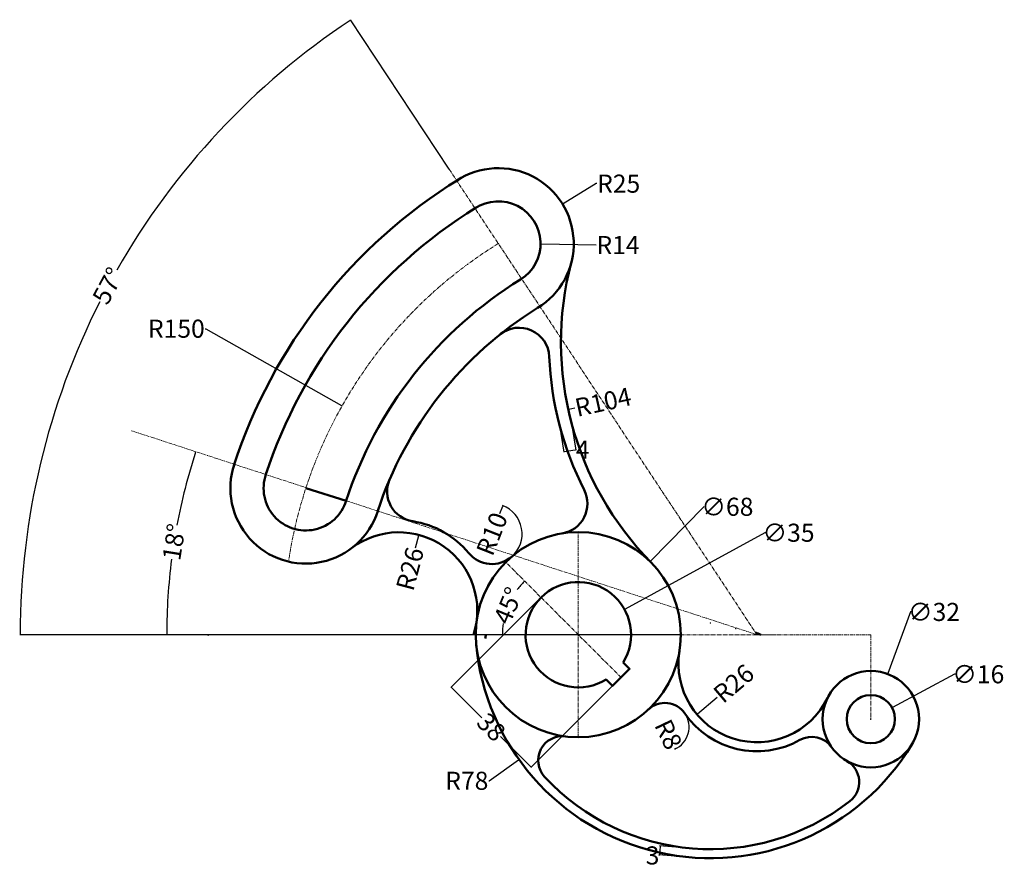
# Model space of a CAD drawing. Units: millimetres. Extents: x -7 to 319, y 85 to 366.
import ezdxf

# ---------------------------------------------------------------- set-up
doc = ezdxf.new("R2010")
doc.units = ezdxf.units.MM
doc.header["$MEASUREMENT"] = 0
doc.linetypes.add('CENTER', pattern=[2, 1.25, -0.25, 0.25, -0.25])
for name, color, linetype, lineweight in [('M-CNTR', 1, 'CENTER', 18), ('M-DIMS', 2, 'Continuous', 25), ('M-OUTL', 7, 'Continuous', 50)]:
    doc.layers.add(name, color=color, linetype=linetype, lineweight=lineweight)
doc.styles.get("Standard").update_dxf_attribs({"font": 'arial.ttf'})
doc.dimstyles.get("Standard").update_dxf_attribs({"dimtxt": 6, "dimasz": 0.18, "dimexe": 0.18, "dimexo": 0.0625, "dimgap": 0.09, "dimtad": 0, "dimtoh": 1, "dimdec": 0, "dimzin": 0, "dimdsep": 46, "dimtxsty": 'Standard', "dimcen": 0.09, "dimadec": 0, "dimazin": 0, "dimtfac": 1, "dimtdec": 0, "dimtofl": 0, "dimtmove": 0, "dimatfit": 3, "dimfxl": 1, "dimtolj": 1, "dimtzin": 0, "dimarcsym": 0})

# ---------------------------------------------------------------- blocks, each defined once
blk = doc.blocks.new('*D1')
at = {"layer": 'Defpoints', "color": 0, "transparency": 16777216}
for p in [(206.85, 131.16), (210.29, 123.94)]:
    blk.add_point(p, dxfattribs=at)
at = {"layer": 'M-DIMS', "color": 0, "lineweight": -2, "transparency": 16777216}
blk.add_line((210.14, 124.27), (210.21, 124.1), dxfattribs=at)
blk.add_arc((206.85, 131.16), 8, 294.21, 34.0846, dxfattribs=at)
at = {"layer": 'M-DIMS', "color": 0, "transparency": 16777216}
blk.add_solid([(210.24, 124.12), (210.19, 124.09), (210.29, 123.94)], dxfattribs=at)
at = {"layer": 'M-DIMS', "color": 0, "transparency": 16777216, "insert": (208.01, 128.72), "char_height": 6, "attachment_point": 5, "rotation": 295.4992}
blk.add_mtext('\\A1;R8', dxfattribs=at)
blk = doc.blocks.new('*D2')
at = {"layer": 'Defpoints', "color": 0, "transparency": 16777216}
for p in [(153.14, 204.52), (149.49, 195.21)]:
    blk.add_point(p, dxfattribs=at)
at = {"layer": 'M-DIMS', "color": 0, "lineweight": -2, "transparency": 16777216}
blk.add_line((152.14, 201.96), (153.08, 204.35), dxfattribs=at)
blk.add_arc((149.49, 195.21), 10, 310.9371, 69.6028, dxfattribs=at)
at = {"layer": 'M-DIMS', "color": 0, "transparency": 16777216}
blk.add_solid([(153.05, 204.36), (153.1, 204.34), (153.14, 204.52)], dxfattribs=at)
at = {"layer": 'M-DIMS', "color": 0, "transparency": 16777216, "insert": (149.49, 195.21), "char_height": 6, "attachment_point": 5, "rotation": 68.5714}
blk.add_mtext('\\A1;R10', dxfattribs=at)
blk = doc.blocks.new('*D3')
at = {"layer": 'Defpoints', "color": 0, "transparency": 16777216}
for p in [(237.33, 152.14), (217.49, 135.33)]:
    blk.add_point(p, dxfattribs=at)
at = {"layer": 'M-DIMS', "color": 0, "lineweight": -2, "transparency": 16777216}
blk.add_line((224.11, 140.94), (217.62, 135.45), dxfattribs=at)
at = {"layer": 'M-DIMS', "color": 0, "transparency": 16777216}
blk.add_solid([(217.6, 135.47), (217.64, 135.43), (217.49, 135.33)], dxfattribs=at)
at = {"layer": 'M-DIMS', "color": 0, "transparency": 16777216, "insert": (229.65, 145.63), "char_height": 6, "attachment_point": 5, "rotation": 40.2578}
blk.add_mtext('\\A1;R26', dxfattribs=at)
blk = doc.blocks.new('*D4')
at = {"layer": 'Defpoints', "color": 0, "transparency": 16777216}
for p in [(221.94, 165.68), (158.45, 120.37)]:
    blk.add_point(p, dxfattribs=at)
at = {"layer": 'M-DIMS', "color": 0, "lineweight": -2, "transparency": 16777216}
for p, q in [((221.85, 165.68), (222.03, 165.68)), ((221.94, 165.59), (221.94, 165.77)), ((148.61, 113.35), (158.3, 120.26)), ((148.43, 113.35), (148.61, 113.35))]:
    blk.add_line(p, q, dxfattribs=at)
at = {"layer": 'M-DIMS', "color": 0, "transparency": 16777216}
blk.add_solid([(158.28, 120.29), (158.32, 120.24), (158.45, 120.37)], dxfattribs=at)
at = {"layer": 'M-DIMS', "color": 0, "transparency": 16777216, "insert": (141.16, 113.35), "char_height": 6, "attachment_point": 5}
blk.add_mtext('\\A1;R78', dxfattribs=at)
blk = doc.blocks.new('*D5')
at = {"layer": 'Defpoints', "color": 0, "transparency": 16777216}
for p in [(125.27, 194.88), (118.64, 169.74)]:
    blk.add_point(p, dxfattribs=at)
at = {"layer": 'M-DIMS', "color": 0, "lineweight": -2, "transparency": 16777216}
blk.add_line((124.15, 190.62), (125.23, 194.71), dxfattribs=at)
at = {"layer": 'M-DIMS', "color": 0, "transparency": 16777216}
blk.add_solid([(125.2, 194.72), (125.26, 194.7), (125.27, 194.88)], dxfattribs=at)
at = {"layer": 'M-DIMS', "color": 0, "transparency": 16777216, "insert": (122.3, 183.6), "char_height": 6, "attachment_point": 5, "rotation": 75.2273}
blk.add_mtext('\\A1;R26', dxfattribs=at)
blk = doc.blocks.new('*D6')
at = {"layer": 'Defpoints', "color": 0, "transparency": 16777216}
for p in [(276.37, 258.69), (174.79, 236.4)]:
    blk.add_point(p, dxfattribs=at)
at = {"layer": 'M-DIMS', "color": 0, "lineweight": -2, "transparency": 16777216}
blk.add_line((176.98, 236.89), (174.96, 236.44), dxfattribs=at)
at = {"layer": 'M-DIMS', "color": 0, "transparency": 16777216}
blk.add_solid([(174.96, 236.47), (174.97, 236.41), (174.79, 236.4)], dxfattribs=at)
at = {"layer": 'M-DIMS', "color": 0, "transparency": 16777216, "insert": (186.34, 238.94), "char_height": 6, "attachment_point": 5, "rotation": 12.3714}
blk.add_mtext('\\A1;R104', dxfattribs=at)
blk = doc.blocks.new('*D7')
at = {"layer": 'Defpoints', "color": 0, "transparency": 16777216}
for p in [(99.82, 237.67), (230.38, 163.83)]:
    blk.add_point(p, dxfattribs=at)
at = {"layer": 'M-DIMS', "color": 0, "lineweight": -2, "transparency": 16777216}
for p, q in [((54.44, 263.24), (54.62, 263.24)), ((54.62, 263.24), (99.66, 237.76)), ((230.29, 163.83), (230.47, 163.83)), ((230.38, 163.74), (230.38, 163.92))]:
    blk.add_line(p, q, dxfattribs=at)
at = {"layer": 'M-DIMS', "color": 0, "transparency": 16777216}
blk.add_solid([(99.68, 237.79), (99.65, 237.74), (99.82, 237.67)], dxfattribs=at)
at = {"layer": 'M-DIMS', "color": 0, "transparency": 16777216, "insert": (44.86, 263.24), "char_height": 6, "attachment_point": 5}
blk.add_mtext('\\A1;R150', dxfattribs=at)
blk = doc.blocks.new('*D8')
at = {"layer": 'Defpoints', "color": 0, "transparency": 16777216}
for p in [(165.73, 174.17), (192.28, 147.62), (162.54, 117.89)]:
    blk.add_point(p, dxfattribs=at)
at = {"layer": 'M-DIMS', "color": 0, "lineweight": -2, "transparency": 16777216}
for p, q in [((165.69, 174.12), (135.87, 144.3)), ((192.23, 147.58), (162.42, 117.76)), ((136.13, 144.3), (146.17, 134.26)), ((162.42, 118.02), (152.38, 128.05))]:
    blk.add_line(p, q, dxfattribs=at)
at = {"layer": 'M-DIMS', "color": 0, "transparency": 16777216}
for points in [[(136.15, 144.32), (136.11, 144.28), (136, 144.43)], [(162.44, 118.04), (162.39, 117.99), (162.54, 117.89)]]:
    blk.add_solid(points, dxfattribs=at)
at = {"layer": 'M-DIMS', "color": 0, "transparency": 16777216, "insert": (149.27, 131.16), "char_height": 6, "attachment_point": 5, "rotation": 315}
blk.add_mtext('\\A1;38', dxfattribs=at)
blk = doc.blocks.new('*D9')
at = {"layer": 'Defpoints', "color": 0, "transparency": 16777216}
for p in [(193.47, 170.18), (162.75, 153.4)]:
    blk.add_point(p, dxfattribs=at)
at = {"layer": 'M-DIMS', "color": 0, "lineweight": -2, "transparency": 16777216}
for p, q in [((239.97, 195.59), (193.62, 170.27)), ((240.15, 195.59), (239.97, 195.59)), ((178.02, 161.79), (178.2, 161.79)), ((178.11, 161.7), (178.11, 161.88))]:
    blk.add_line(p, q, dxfattribs=at)
at = {"layer": 'M-DIMS', "color": 0, "transparency": 16777216}
blk.add_solid([(193.61, 170.29), (193.64, 170.24), (193.47, 170.18)], dxfattribs=at)
at = {"layer": 'M-DIMS', "color": 0, "transparency": 16777216, "insert": (247.82, 195.59), "char_height": 6, "attachment_point": 5}
blk.add_mtext('\\A1;∅35', dxfattribs=at)
blk = doc.blocks.new('*D10')
at = {"layer": 'Defpoints', "color": 0, "transparency": 16777216}
for p in [(201.92, 186.06), (154.3, 137.52)]:
    blk.add_point(p, dxfattribs=at)
at = {"layer": 'M-DIMS', "color": 0, "lineweight": -2, "transparency": 16777216}
for p, q in [((219.71, 204.2), (202.04, 186.19)), ((219.89, 204.2), (219.71, 204.2)), ((178.02, 161.79), (178.2, 161.79)), ((178.11, 161.7), (178.11, 161.88))]:
    blk.add_line(p, q, dxfattribs=at)
at = {"layer": 'M-DIMS', "color": 0, "transparency": 16777216}
blk.add_solid([(202.02, 186.21), (202.07, 186.17), (201.92, 186.06)], dxfattribs=at)
at = {"layer": 'M-DIMS', "color": 0, "transparency": 16777216, "insert": (227.54, 204.2), "char_height": 6, "attachment_point": 5}
blk.add_mtext('\\A1;∅68', dxfattribs=at)
blk = doc.blocks.new('*D11')
at = {"layer": 'Defpoints', "color": 0, "transparency": 16777216}
for p in [(282.16, 137.57), (268.06, 130.02)]:
    blk.add_point(p, dxfattribs=at)
at = {"layer": 'M-DIMS', "color": 0, "lineweight": -2, "transparency": 16777216}
for p, q in [((302.9, 148.67), (282.32, 137.65)), ((303.08, 148.67), (302.9, 148.67)), ((275.11, 133.7), (275.11, 133.88)), ((275.02, 133.79), (275.2, 133.79))]:
    blk.add_line(p, q, dxfattribs=at)
at = {"layer": 'M-DIMS', "color": 0, "transparency": 16777216}
blk.add_solid([(282.31, 137.68), (282.34, 137.63), (282.16, 137.57)], dxfattribs=at)
at = {"layer": 'M-DIMS', "color": 0, "transparency": 16777216, "insert": (310.73, 148.67), "char_height": 6, "attachment_point": 5}
blk.add_mtext('\\A1;∅16', dxfattribs=at)
blk = doc.blocks.new('*D12')
at = {"layer": 'Defpoints', "color": 0, "transparency": 16777216}
for p in [(280.66, 148.8), (269.56, 118.78)]:
    blk.add_point(p, dxfattribs=at)
at = {"layer": 'M-DIMS', "color": 0, "lineweight": -2, "transparency": 16777216}
for p, q in [((288.24, 169.33), (280.72, 148.97)), ((288.42, 169.33), (288.24, 169.33)), ((275.11, 133.7), (275.11, 133.88)), ((275.02, 133.79), (275.2, 133.79))]:
    blk.add_line(p, q, dxfattribs=at)
at = {"layer": 'M-DIMS', "color": 0, "transparency": 16777216}
blk.add_solid([(280.69, 148.98), (280.75, 148.96), (280.66, 148.8)], dxfattribs=at)
at = {"layer": 'M-DIMS', "color": 0, "transparency": 16777216, "insert": (296.04, 169.33), "char_height": 6, "attachment_point": 5}
blk.add_mtext('\\A1;∅32', dxfattribs=at)
blk = doc.blocks.new('*D13')
at = {"layer": 'Defpoints', "color": 0, "transparency": 16777216}
for p in [(172.93, 304.53), (151.61, 291.48)]:
    blk.add_point(p, dxfattribs=at)
at = {"layer": 'M-DIMS', "color": 0, "lineweight": -2, "transparency": 16777216}
for p, q in [((184.05, 311.33), (173.09, 304.62)), ((184.23, 311.33), (184.05, 311.33)), ((151.52, 291.48), (151.7, 291.48)), ((151.61, 291.39), (151.61, 291.57))]:
    blk.add_line(p, q, dxfattribs=at)
at = {"layer": 'M-DIMS', "color": 0, "transparency": 16777216}
blk.add_solid([(173.07, 304.65), (173.1, 304.59), (172.93, 304.53)], dxfattribs=at)
at = {"layer": 'M-DIMS', "color": 0, "transparency": 16777216, "insert": (191.51, 311.33), "char_height": 6, "attachment_point": 5}
blk.add_mtext('\\A1;R25', dxfattribs=at)
blk = doc.blocks.new('*D14')
at = {"layer": 'Defpoints', "color": 0, "transparency": 16777216}
for p in [(151.61, 291.48), (165.61, 291.26)]:
    blk.add_point(p, dxfattribs=at)
at = {"layer": 'M-DIMS', "color": 0, "lineweight": -2, "transparency": 16777216}
for p, q in [((151.52, 291.48), (151.7, 291.48)), ((151.61, 291.39), (151.61, 291.57)), ((184.05, 290.98), (165.79, 291.26))]:
    blk.add_line(p, q, dxfattribs=at)
at = {"layer": 'M-DIMS', "color": 0, "transparency": 16777216}
blk.add_solid([(165.79, 291.29), (165.79, 291.23), (165.61, 291.26)], dxfattribs=at)
at = {"layer": 'M-DIMS', "color": 0, "transparency": 16777216, "insert": (191.29, 290.98), "char_height": 6, "attachment_point": 5}
blk.add_mtext('\\A1;R14', dxfattribs=at)
blk = doc.blocks.new('*D15')
at = {"layer": 'Defpoints', "color": 0, "transparency": 16777216}
for p in [(154.07, 185.83), (156.32, 174.37), (28.11, 161.79), (212.11, 161.79), (192.28, 147.62)]:
    blk.add_point(p, dxfattribs=at)
at = {"layer": 'M-DIMS', "color": 0, "lineweight": -2, "transparency": 16777216}
for start, end in [(135.41, 143.4751), (171.5249, 179.59)]:
    blk.add_arc((178.11, 161.79), 25.16, start, end, dxfattribs=at)
at = {"layer": 'M-DIMS', "color": 0, "transparency": 16777216}
for points in [[(160.17, 179.47), (160.22, 179.43), (160.32, 179.58)], [(152.98, 161.97), (152.92, 161.97), (152.95, 161.79)]]:
    blk.add_solid(points, dxfattribs=at)
at = {"layer": 'M-DIMS', "color": 0, "transparency": 16777216, "insert": (154.87, 171.42), "char_height": 6, "attachment_point": 5, "rotation": 67.5}
blk.add_mtext('\\A1;45°', dxfattribs=at)
blk = doc.blocks.new('*D16')
at = {"layer": 'Defpoints', "color": 0, "transparency": 16777216}
for p in [(30, 229.41), (45.95, 202.62), (212.11, 161.79), (237.33, 161.79), (275.11, 161.79)]:
    blk.add_point(p, dxfattribs=at)
at = {"layer": 'M-DIMS', "color": 0, "lineweight": -2, "transparency": 16777216}
blk.add_line((212.05, 161.79), (41.47, 161.79), dxfattribs=at)
for start, end in [(161.9882, 169.3006), (172.6349, 179.9473)]:
    blk.add_arc((237.33, 161.79), 195.68, start, end, dxfattribs=at)
at = {"layer": 'M-DIMS', "color": 0, "transparency": 16777216}
for points in [[(51.21, 222.31), (51.26, 222.29), (51.29, 222.47)], [(41.68, 161.97), (41.62, 161.97), (41.65, 161.79)]]:
    blk.add_solid(points, dxfattribs=at)
at = {"layer": 'M-DIMS', "color": 0, "transparency": 16777216, "insert": (44.07, 192.51), "char_height": 6, "attachment_point": 5, "rotation": 80.9678}
blk.add_mtext('\\A1;18°', dxfattribs=at)
blk = doc.blocks.new('*D17')
at = {"layer": 'Defpoints', "color": 0, "transparency": 16777216}
for p in [(135.34, 316.08), (44.06, 311.12), (212.11, 161.79), (237.33, 161.79), (275.11, 161.79)]:
    blk.add_point(p, dxfattribs=at)
at = {"layer": 'M-DIMS', "color": 0, "lineweight": -2, "transparency": 16777216}
for p, q in [((135.31, 316.14), (102.55, 365.69)), ((212.05, 161.79), (-7.09, 161.79))]:
    blk.add_line(p, q, dxfattribs=at)
for start, end in [(123.5066, 150.3303), (153.1341, 179.9578)]:
    blk.add_arc((237.33, 161.79), 244.24, start, end, dxfattribs=at)
at = {"layer": 'M-DIMS', "color": 0, "transparency": 16777216}
for points in [[(102.49, 365.47), (102.52, 365.42), (102.65, 365.54)], [(-6.88, 161.97), (-6.94, 161.97), (-6.91, 161.79)]]:
    blk.add_solid(points, dxfattribs=at)
at = {"layer": 'M-DIMS', "color": 0, "transparency": 16777216, "insert": (22.22, 277.46), "char_height": 6, "attachment_point": 5, "rotation": 61.7322}
blk.add_mtext('\\A1;57°', dxfattribs=at)
blk = doc.blocks.new('*D18')
at = {"layer": 'Defpoints', "color": 0, "transparency": 16777216}
for p in [(204.99, 88.78), (215.99, 90.91), (215.75, 87.92)]:
    blk.add_point(p, dxfattribs=at)
at = {"layer": 'M-DIMS', "color": 0, "lineweight": -2, "transparency": 16777216}
for p, q in [((205.21, 91.59), (205, 88.96)), ((215.92, 90.92), (205.04, 91.78)), ((204.97, 88.6), (204.79, 88.6)), ((215.69, 87.93), (204.81, 88.79)), ((204.99, 88.78), (204.97, 88.6))]:
    blk.add_line(p, q, dxfattribs=at)
at = {"layer": 'M-DIMS', "color": 0, "transparency": 16777216}
for points in [[(205.18, 91.59), (205.24, 91.59), (205.22, 91.77)], [(204.97, 88.96), (205.03, 88.96), (204.99, 88.78)]]:
    blk.add_solid(points, dxfattribs=at)
at = {"layer": 'M-DIMS', "color": 0, "transparency": 16777216, "insert": (202.74, 88.6), "char_height": 6, "attachment_point": 5}
blk.add_mtext('\\A1;3', dxfattribs=at)
blk = doc.blocks.new('*D19')
at = {"layer": 'Defpoints', "color": 0, "transparency": 16777216}
for p in [(175.88, 231.88), (171.91, 231.27), (177.23, 223.12)]:
    blk.add_point(p, dxfattribs=at)
at = {"layer": 'M-DIMS', "color": 0, "lineweight": -2, "transparency": 16777216}
for p, q in [((175.89, 231.82), (177.26, 222.94)), ((171.92, 231.21), (173.28, 222.33)), ((173.43, 222.54), (177.05, 223.09)), ((177.23, 223.12), (177.41, 223.15))]:
    blk.add_line(p, q, dxfattribs=at)
at = {"layer": 'M-DIMS', "color": 0, "transparency": 16777216}
for points in [[(173.43, 222.57), (173.44, 222.51), (173.26, 222.51)], [(177.05, 223.12), (177.06, 223.06), (177.23, 223.12)]]:
    blk.add_solid(points, dxfattribs=at)
at = {"layer": 'M-DIMS', "color": 0, "transparency": 16777216, "insert": (179.58, 223.15), "char_height": 6, "attachment_point": 5}
blk.add_mtext('\\A1;4', dxfattribs=at)

msp = doc.modelspace()

# ---------------------------------------------------------------- linework, layer by layer
at = {"layer": 'M-CNTR'}
for p, q in [((118.33, 195.74), (118.33, 195.79)), ((178.11, 127.79), (178.11, 195.79)), ((192.28, 147.62), (154.07, 185.83)), ((243.61, 161.79), (237.33, 161.79)), ((204.98, 140.58), (204.81, 140.74)), ((199.32, 134.92), (199.16, 135.09))]:
    msp.add_line(p, q, dxfattribs=at)
for points in [[(135.34, 316.08), (237.33, 161.79), (30, 229.41)], [(28.11, 161.79), (212.11, 161.79), (275.11, 161.79), (275.11, 133.79)]]:
    msp.add_lwpolyline(points, dxfattribs=at)
msp.add_lwpolyline([(66.4, 161.79, 0.00029), (66.4, 161.6, -0.00029)], format="xyb", close=True, dxfattribs=at)
for radius, start, end in [(164, 121.6794, 161.9355), (164, 121.6794, 161.9355), (164, 121.6794, 161.9355), (150, 121.6794, 171.4959), (175, 180.6665, 180.7776), (164, 180.7112, 180.7776), (164, 180.7112, 180.7776), (164, 180.7112, 180.7776), (164, 180.7112, 180.7776)]:
    msp.add_arc((230.38, 163.83), radius, start, end, dxfattribs=at)
at = {"layer": 'M-OUTL'}
for points in [[(111.61, 202.8, -0.17665), (164.58, 270.11, 1.019438), (137.82, 312.33)], [(101.09, 206, -0.177479), (158.96, 279.56, 1.015699), (143.89, 303.16)], [(172.75, 195.37, 0.508734), (180.08, 209.77, -0.107095), (168.47, 254.01, 0.61411), (152.23, 261.38)], [(87.78, 210.34), (101.15, 206.21, -1.015734), (74.54, 214.89)], [(115.56, 213.23, 0.490469), (123.22, 199.39, -0.183903), (141.78, 188.84, 0.4195), (155.99, 187.61)], [(262.05, 124.54, 0.384618), (251.59, 126.88, -0.388513), (213.44, 135.7, 0.459113), (201.37, 137)], [(173.81, 128.06, 0.700795), (166.94, 114.69, 0.390052), (268.18, 106.63, 0.533462), (267.2, 119.88)]]:
    msp.add_lwpolyline(points, format="xyb", dxfattribs=at)
msp.add_lwpolyline([(192.98, 152.57), (195.11, 150.45), (189.45, 144.79), (187.33, 146.92, -8.634181)], format="xyb", close=True, dxfattribs=at)
for centre, radius in [((178.11, 161.79), 34), ((275.11, 133.79), 16), ((275.11, 133.79), 8)]:
    msp.add_circle(centre, radius, dxfattribs=at)
for centre, radius, start, end in [((230.38, 163.83), 175, 121.6794, 162.0067), ((230.38, 163.83), 164, 121.6794, 161.9355), ((276.37, 258.69), 104, 165.2743, 224.5988), ((87.78, 210.34), 25, 161.4346, 342.4364), ((118.64, 169.74), 26, 342.1953, 127.2497), ((118.64, 169.74), 30, 342.1953, 344.6328), ((276.37, 258.69), 104, 247.681, 248.6987), ((221.94, 165.68), 78, 185.0674, 329.0496), ((237.33, 152.14), 26, 170.7394, 334.1018)]:
    msp.add_arc(centre, radius, start, end, dxfattribs=at)

# ---------------------------------------------------------------- dimensions: what is measured, and where the dimension line sits
at = {"layer": 'M-DIMS'}
for base, line1, line2, picture, middle in [((44.06, 311.12), ((212.11, 161.79), (275.11, 161.79)), ((135.34, 316.08), (237.33, 161.79)), '*D17', (22.22, 277.46)), ((45.95, 202.62), ((212.11, 161.79), (275.11, 161.79)), ((237.33, 161.79), (30, 229.41)), '*D16', (44.07, 192.51)), ((156.32, 174.37), ((28.11, 161.79), (212.11, 161.79)), ((192.28, 147.62), (154.07, 185.83)), '*D15', (154.87, 171.42))]:
    dim = msp.add_angular_dim_2l(base=base, line1=line1, line2=line2, dimstyle='Standard', override={"dimclrd": 0, "dimclre": 0, "dimclrt": 0}, dxfattribs=at)
    dim.commit()
    dim.dimension.update_dxf_attribs({"geometry": picture, "text_midpoint": middle})
for center, mpoint, picture, middle in [((151.61, 291.48), (172.93, 304.53), '*D13', (191.51, 311.33)), ((151.61, 291.48), (165.61, 291.26), '*D14', (184.05, 290.98)), ((230.38, 163.83), (99.82, 237.67), '*D7', (44.86, 263.24)), ((276.37, 258.69), (174.79, 236.4), '*D6', (186.34, 238.94)), ((149.49, 195.21), (153.14, 204.52), '*D2', (149.49, 195.21)), ((118.64, 169.74), (125.27, 194.88), '*D5', (122.3, 183.6)), ((221.94, 165.68), (158.45, 120.37), '*D4', (141.16, 113.35)), ((237.33, 152.14), (217.49, 135.33), '*D3', (229.65, 145.63)), ((206.85, 131.16), (210.29, 123.94), '*D1', (208.01, 128.72))]:
    dim = msp.add_radius_dim(center=center, mpoint=mpoint, dimstyle='Standard', override={"dimclrd": 0, "dimclre": 0, "dimclrt": 0}, dxfattribs=at)
    dim.commit()
    dim.dimension.update_dxf_attribs({"geometry": picture, "text_midpoint": middle, "dimtype": 164})
for p1, p2, distance, picture, middle in [((171.91, 231.27), (175.88, 231.88), -8.86, '*D19', (179.58, 223.15)), ((165.73, 174.17), (192.28, 147.62), -42.05, '*D8', (149.27, 131.16)), ((215.99, 90.91), (215.75, 87.92), -10.8, '*D18', (202.74, 88.6))]:
    dim = msp.add_aligned_dim(p1=p1, p2=p2, distance=distance, dimstyle='Standard', override={"dimclrd": 0, "dimclre": 0, "dimclrt": 0}, dxfattribs=at)
    dim.commit()
    dim.dimension.update_dxf_attribs({"geometry": picture, "text_midpoint": middle})
for p1, p2, picture, middle in [((154.3, 137.52), (201.92, 186.06), '*D10', (227.54, 204.2)), ((162.75, 153.4), (193.47, 170.18), '*D9', (247.82, 195.59)), ((269.56, 118.78), (280.66, 148.8), '*D12', (296.04, 169.33)), ((268.06, 130.02), (282.16, 137.57), '*D11', (310.73, 148.67))]:
    dim = msp.add_diameter_dim_2p(p1=p1, p2=p2, dimstyle='Standard', override={"dimclrd": 0, "dimclre": 0, "dimclrt": 0}, dxfattribs=at)
    dim.commit()
    dim.dimension.update_dxf_attribs({"geometry": picture, "text_midpoint": middle, "dimtype": 163})

doc.saveas('drawing.dxf')
